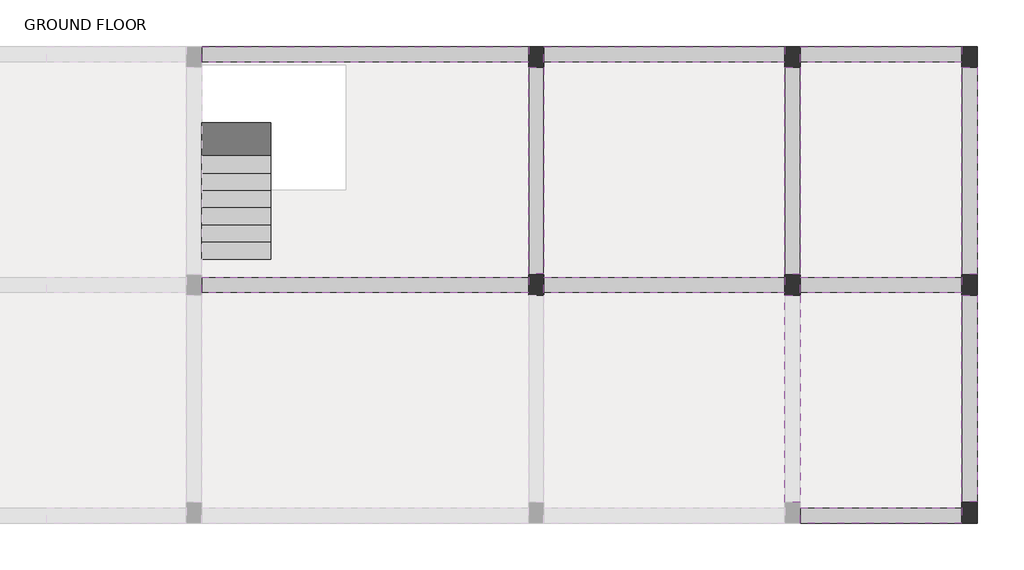
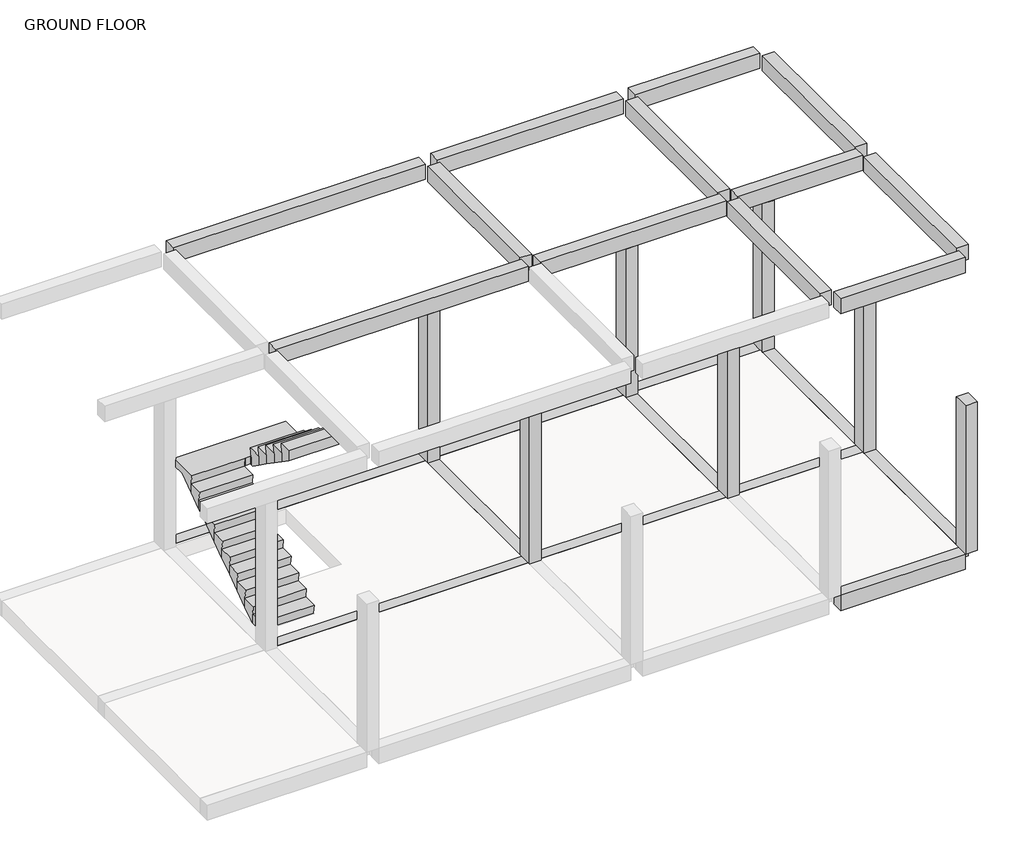
# One storey, part 2 of 2: 23 beams, 7 columns, 1 stair flight.
"""IFC4 building model written with IfcOpenShell, lengths in millimetres."""

from ifc_helpers import new_model, si_unit, frame, origin, place, context, project, spatial, polyline, outline, extrude, faceted_brep, element, save

model = new_model("IFC4")

# Units and contexts
model_context = context("Model", 3, world=origin())
ifc_project = project(units=[si_unit("LENGTHUNIT", "METRE", prefix="MILLI")], contexts=[model_context])

# Site, building, storey
site = spatial("IfcSite", under=ifc_project)
building = spatial("IfcBuilding", under=site)
storey = spatial("IfcBuildingStorey", under=building, Name="GROUND FLOOR", Elevation=0.0)

# Beams
placement = place(None, origin())
element("IfcBeam", 1, ObjectType="M_Concrete-Rectangular Beam : 100MM X 200MM", at=placement, inside=storey, context=model_context, shape_type="Brep", body=[
    faceted_brep([(9387.3931183, 2041.8765586, 0.0), (9387.3931183, 2270.4765586, 0.0), (7001.6931183, 2270.4765586, 0.0), (7001.6931183, 2041.8765586, 0.0), (9387.3931183, 2041.8765586, -304.8), (7001.6931183, 2041.8765586, -304.8), (9387.3931183, 2270.4765586, -304.8), (7001.6931183, 2270.4765586, -304.8), (7001.6931183, 2270.4765586, -300.0)], [[[0, 1, 2, 3]], [[4, 0, 3, 5]], [[6, 4, 5, 7]], [[1, 6, 7, 8, 2]], [[1, 0, 4, 6]], [[3, 2, 8, 7, 5]]]),
])
element("IfcBeam", 2, ObjectType="M_Concrete-Rectangular Beam : 100MM X 200MM", at=placement, inside=storey, context=model_context, shape_type="Brep", body=[
    faceted_brep([(2988.4931183, 8849.0765586, 0.0), (2988.4931183, 9077.6765586, 0.0), (-1837.5068817, 9077.6765586, 0.0), (-1837.5068817, 8849.0765586, 0.0), (2988.4931183, 8849.0765586, -304.8), (2988.4931183, 8849.0765586, -300.0), (-1837.5068817, 8849.0765586, -300.0), (-1837.5068817, 8849.0765586, -304.8), (2988.4931183, 9077.6765586, -304.8), (-1837.5068817, 9077.6765586, -304.8)], [[[0, 1, 2, 3]], [[4, 5, 0, 3, 6, 7]], [[8, 4, 7, 9]], [[1, 8, 9, 2]], [[1, 0, 5, 4, 8]], [[3, 2, 9, 7, 6]]]),
])
element("IfcBeam", 3, ObjectType="M_Concrete-Rectangular Beam : 100MM X 200MM", at=placement, inside=storey, context=model_context, shape_type="Brep", body=[
    faceted_brep([(6773.0931183, 8849.0765586, 0.0), (6773.0931183, 9077.6765586, 0.0), (3217.0931183, 9077.6765586, 0.0), (3217.0931183, 8849.0765586, 0.0), (6773.0931183, 8849.0765586, -304.8), (6773.0931183, 8849.0765586, -300.0), (3217.0931183, 8849.0765586, -300.0), (3217.0931183, 8849.0765586, -304.8), (6773.0931183, 9077.6765586, -304.8), (3217.0931183, 9077.6765586, -304.8)], [[[0, 1, 2, 3]], [[4, 5, 0, 3, 6, 7]], [[8, 4, 7, 9]], [[1, 8, 9, 2]], [[1, 0, 5, 4, 8]], [[3, 2, 9, 7, 6]]]),
])
element("IfcBeam", 4, ObjectType="M_Concrete-Rectangular Beam : 100MM X 200MM", at=placement, inside=storey, context=model_context, shape_type="Brep", body=[
    faceted_brep([(9387.3931183, 8849.0765586, 0.0), (9387.3931183, 9077.6765586, 0.0), (7001.6931183, 9077.6765586, 0.0), (7001.6931183, 8849.0765586, 0.0), (9387.3931183, 8849.0765586, -304.8), (7001.6931183, 8849.0765586, -300.0), (7001.6931183, 8849.0765586, -304.8), (9387.3931183, 9077.6765586, -304.8), (7001.6931183, 9077.6765586, -304.8)], [[[0, 1, 2, 3]], [[4, 0, 3, 5, 6]], [[7, 4, 6, 8]], [[1, 7, 8, 2]], [[1, 0, 4, 7]], [[3, 2, 8, 6, 5]]]),
])
element("IfcBeam", 5, ObjectType="M_Concrete-Rectangular Beam : 100MM X 200MM", at=placement, inside=storey, context=model_context, shape_type="SweptSolid", body=[
    extrude(outline(polyline([(9617.8931183, 2354.2765586), (9389.2931183, 2354.2765586), (9389.2931183, 5407.2180792), (9617.8931183, 5407.2180792), (9617.8931183, 2354.2765586)])), frame((0.0, 0.0, -304.8), z_axis=(0.0, 0.0, 1.0), x_axis=(1.0, 0.0, 0.0)), (0.0, 0.0, 1.0), 304.8),
])
element("IfcBeam", 6, ObjectType="M_Concrete-Rectangular Beam : 100MM X 200MM", at=placement, inside=storey, context=model_context, shape_type="SweptSolid", body=[
    extrude(outline(polyline([(9389.2931183, 8772.8765586), (9617.8931183, 8772.8765586), (9617.8931183, 5712.0180792), (9389.2931183, 5712.0180792), (9389.2931183, 8772.8765586)])), frame((0.0, 0.0, -304.8), z_axis=(0.0, 0.0, 1.0), x_axis=(1.0, 0.0, 0.0)), (0.0, 0.0, 1.0), 304.8),
])
element("IfcBeam", 7, ObjectType="M_Concrete-Rectangular Beam : 100MM X 200MM", at=placement, inside=storey, context=model_context, shape_type="Brep", body=[
    faceted_brep([(9389.2931183, 5445.3180792, 0.0), (9389.2931183, 5673.9180792, 0.0), (7001.6931183, 5673.9180792, 0.0), (7001.6931183, 5445.3180792, 0.0), (9389.2931183, 5673.9180792, -300.0), (9389.2931183, 5673.9180792, -304.8), (7001.6931183, 5673.9180792, -304.8), (7001.6931183, 5673.9180792, -300.0), (9389.2931183, 5445.3180792, -304.8), (7001.6931183, 5445.3180792, -304.8), (7001.6931183, 5445.3180792, -300.0), (9389.2931183, 5445.3180792, -300.0)], [[[0, 1, 2, 3]], [[2, 1, 4, 5, 6, 7]], [[5, 8, 9, 6]], [[0, 3, 10, 9, 8, 11]], [[1, 0, 11, 8, 5, 4]], [[3, 2, 7, 6, 9, 10]]]),
])
element("IfcBeam", 8, ObjectType="M_Concrete-Rectangular Beam : 100MM X 200MM", at=placement, inside=storey, context=model_context, shape_type="Brep", body=[
    faceted_brep([(6773.0931183, 5445.3180792, 0.0), (6773.0931183, 5673.9180792, 0.0), (3217.0931183, 5673.9180792, 0.0), (3217.0931183, 5445.3180792, 0.0), (6773.0931183, 5673.9180792, -300.0), (6773.0931183, 5673.9180792, -304.8), (3217.0931183, 5673.9180792, -304.8), (3217.0931183, 5673.9180792, -300.0), (6773.0931183, 5445.3180792, -304.8), (3217.0931183, 5445.3180792, -304.8), (3217.0931183, 5445.3180792, -300.0), (6773.0931183, 5445.3180792, -300.0)], [[[0, 1, 2, 3]], [[2, 1, 4, 5, 6, 7]], [[5, 8, 9, 6]], [[0, 3, 10, 9, 8, 11]], [[1, 0, 11, 8, 5, 4]], [[3, 2, 7, 6, 9, 10]]]),
])
element("IfcBeam", 9, ObjectType="M_Concrete-Rectangular Beam : 100MM X 200MM", at=placement, inside=storey, context=model_context, shape_type="Brep", body=[
    faceted_brep([(2988.4931183, 5445.3180792, 0.0), (2988.4931183, 5673.9180792, 0.0), (-1837.5068817, 5673.9180792, 0.0), (-1837.5068817, 5445.3180792, 0.0), (2988.4931183, 5673.9180792, -300.0), (2988.4931183, 5673.9180792, -304.8), (-1837.5068817, 5673.9180792, -304.8), (-1837.5068817, 5673.9180792, -300.0), (2988.4931183, 5445.3180792, -304.8), (-1837.5068817, 5445.3180792, -304.8), (-1837.5068817, 5445.3180792, -300.0), (2988.4931183, 5445.3180792, -300.0)], [[[0, 1, 2, 3]], [[2, 1, 4, 5, 6, 7]], [[5, 8, 9, 6]], [[0, 3, 10, 9, 8, 11]], [[1, 0, 11, 8, 5, 4]], [[3, 2, 7, 6, 9, 10]]]),
])
element("IfcBeam", 10, ObjectType="M_Concrete-Rectangular Beam : 100MM X 200MM", at=placement, inside=storey, context=model_context, shape_type="Brep", body=[
    faceted_brep([(7001.6931183, 8772.8765586, 0.0), (6773.0931183, 8772.8765586, 0.0), (6773.0931183, 5712.0180792, 0.0), (7001.6931183, 5712.0180792, 0.0), (7001.6931183, 5712.0180792, -300.0), (7001.6931183, 5712.0180792, -304.8), (7001.6931183, 8772.8765586, -304.8), (7001.6931183, 8772.8765586, -300.0), (6773.0931183, 8772.8765586, -304.8), (6773.0931183, 5712.0180792, -304.8), (6773.0931183, 8772.8765586, -300.0), (6773.0931183, 5712.0180792, -300.0)], [[[0, 1, 2, 3]], [[0, 3, 4, 5, 6, 7]], [[8, 6, 5, 9]], [[2, 1, 10, 8, 9, 11]], [[1, 0, 7, 6, 8, 10]], [[3, 2, 11, 9, 5, 4]]]),
])
element("IfcBeam", 11, ObjectType="M_Concrete-Rectangular Beam : 100MM X 200MM", at=placement, inside=storey, context=model_context, shape_type="Brep", body=[
    faceted_brep([(2988.4931183, 5719.6180792, 0.0), (3217.0931183, 5719.6180792, 0.0), (3217.0931183, 8772.8765586, 0.0), (2988.4931183, 8772.8765586, 0.0), (3217.0931183, 5719.6180792, -300.0), (3217.0931183, 5719.6180792, -304.8), (3217.0931183, 8772.8765586, -304.8), (3217.0931183, 8772.8765586, -300.0), (2988.4931183, 5719.6180792, -304.8), (2988.4931183, 8772.8765586, -304.8), (2988.4931183, 8772.8765586, -300.0), (2988.4931183, 5719.6180792, -300.0)], [[[0, 1, 2, 3]], [[2, 1, 4, 5, 6, 7]], [[5, 8, 9, 6]], [[0, 3, 10, 9, 8, 11]], [[8, 5, 4, 1, 0, 11]], [[3, 2, 7, 6, 9, 10]]]),
])
element("IfcBeam", 12, ObjectType="M_Concrete-Rectangular Beam : 100MM X 200MM", at=placement, inside=storey, context=model_context, shape_type="Brep", body=[
    faceted_brep([(9387.3931183, 2041.8765586, 6000.0), (9387.3931183, 2270.4765586, 6000.0), (7001.6931183, 2270.4765586, 6000.0), (7001.6931183, 2041.8765586, 6000.0), (9387.3931183, 2041.8765586, 5695.2), (7001.6931183, 2041.8765586, 5695.2), (9387.3931183, 2270.4765586, 5695.2), (7001.6931183, 2270.4765586, 5695.2), (7001.6931183, 2270.4765586, 5700.0)], [[[0, 1, 2, 3]], [[4, 0, 3, 5]], [[6, 4, 5, 7]], [[1, 6, 7, 8, 2]], [[1, 0, 4, 6]], [[3, 2, 8, 7, 5]]]),
])
element("IfcBeam", 13, ObjectType="M_Concrete-Rectangular Beam : 100MM X 200MM", at=placement, inside=storey, context=model_context, shape_type="Brep", body=[
    faceted_brep([(2988.4931183, 8849.0765586, 6000.0), (2988.4931183, 9077.6765586, 6000.0), (-1837.5068817, 9077.6765586, 6000.0), (-1837.5068817, 8849.0765586, 6000.0), (2988.4931183, 8849.0765586, 5695.2), (2988.4931183, 8849.0765586, 5700.0), (-1837.5068817, 8849.0765586, 5700.0), (-1837.5068817, 8849.0765586, 5695.2), (2988.4931183, 9077.6765586, 5695.2), (-1837.5068817, 9077.6765586, 5695.2)], [[[0, 1, 2, 3]], [[4, 5, 0, 3, 6, 7]], [[8, 4, 7, 9]], [[1, 8, 9, 2]], [[1, 0, 5, 4, 8]], [[3, 2, 9, 7, 6]]]),
])
element("IfcBeam", 14, ObjectType="M_Concrete-Rectangular Beam : 100MM X 200MM", at=placement, inside=storey, context=model_context, shape_type="Brep", body=[
    faceted_brep([(6773.0931183, 8849.0765586, 6000.0), (6773.0931183, 9077.6765586, 6000.0), (3217.0931183, 9077.6765586, 6000.0), (3217.0931183, 8849.0765586, 6000.0), (6773.0931183, 8849.0765586, 5695.2), (6773.0931183, 8849.0765586, 5700.0), (3217.0931183, 8849.0765586, 5700.0), (3217.0931183, 8849.0765586, 5695.2), (6773.0931183, 9077.6765586, 5695.2), (3217.0931183, 9077.6765586, 5695.2)], [[[0, 1, 2, 3]], [[4, 5, 0, 3, 6, 7]], [[8, 4, 7, 9]], [[1, 8, 9, 2]], [[1, 0, 5, 4, 8]], [[3, 2, 9, 7, 6]]]),
])
element("IfcBeam", 15, ObjectType="M_Concrete-Rectangular Beam : 100MM X 200MM", at=placement, inside=storey, context=model_context, shape_type="Brep", body=[
    faceted_brep([(9387.3931183, 8849.0765586, 6000.0), (9387.3931183, 9077.6765586, 6000.0), (7001.6931183, 9077.6765586, 6000.0), (7001.6931183, 8849.0765586, 6000.0), (9387.3931183, 8849.0765586, 5695.2), (7001.6931183, 8849.0765586, 5700.0), (7001.6931183, 8849.0765586, 5695.2), (9387.3931183, 9077.6765586, 5695.2), (7001.6931183, 9077.6765586, 5695.2)], [[[0, 1, 2, 3]], [[4, 0, 3, 5, 6]], [[7, 4, 6, 8]], [[1, 7, 8, 2]], [[1, 0, 4, 7]], [[3, 2, 8, 6, 5]]]),
])
element("IfcBeam", 16, ObjectType="M_Concrete-Rectangular Beam : 100MM X 200MM", at=placement, inside=storey, context=model_context, shape_type="SweptSolid", body=[
    extrude(outline(polyline([(9617.8931183, 2354.2765586), (9389.2931183, 2354.2765586), (9389.2931183, 5407.2180792), (9617.8931183, 5407.2180792), (9617.8931183, 2354.2765586)])), frame((0.0, 0.0, 5695.2), z_axis=(0.0, 0.0, 1.0), x_axis=(1.0, 0.0, 0.0)), (0.0, 0.0, 1.0), 304.8),
])
element("IfcBeam", 17, ObjectType="M_Concrete-Rectangular Beam : 100MM X 200MM", at=placement, inside=storey, context=model_context, shape_type="SweptSolid", body=[
    extrude(outline(polyline([(9389.2931183, 8772.8765586), (9617.8931183, 8772.8765586), (9617.8931183, 5712.0180792), (9389.2931183, 5712.0180792), (9389.2931183, 8772.8765586)])), frame((0.0, 0.0, 5695.2), z_axis=(0.0, 0.0, 1.0), x_axis=(1.0, 0.0, 0.0)), (0.0, 0.0, 1.0), 304.8),
])
element("IfcBeam", 18, ObjectType="M_Concrete-Rectangular Beam : 100MM X 200MM", at=placement, inside=storey, context=model_context, shape_type="Brep", body=[
    faceted_brep([(7001.6931183, 5445.3180792, 6000.0), (9389.2931183, 5445.3180792, 6000.0), (9389.2931183, 5673.9180792, 6000.0), (7001.6931183, 5673.9180792, 6000.0), (9389.2931183, 5673.9180792, 5700.0), (9389.2931183, 5673.9180792, 5695.2), (7001.6931183, 5673.9180792, 5695.2), (7001.6931183, 5673.9180792, 5700.0), (9389.2931183, 5445.3180792, 5695.2), (7001.6931183, 5445.3180792, 5695.2), (7001.6931183, 5445.3180792, 5700.0), (9389.2931183, 5445.3180792, 5700.0)], [[[0, 1, 2, 3]], [[3, 2, 4, 5, 6, 7]], [[5, 8, 9, 6]], [[1, 0, 10, 9, 8, 11]], [[5, 4, 2, 1, 11, 8]], [[0, 3, 7, 6, 9, 10]]]),
])
element("IfcBeam", 19, ObjectType="M_Concrete-Rectangular Beam : 100MM X 200MM", at=placement, inside=storey, context=model_context, shape_type="Brep", body=[
    faceted_brep([(3217.0931183, 5445.3180792, 6000.0), (6773.0931183, 5445.3180792, 6000.0), (6773.0931183, 5673.9180792, 6000.0), (3217.0931183, 5673.9180792, 6000.0), (6773.0931183, 5673.9180792, 5700.0), (6773.0931183, 5673.9180792, 5695.2), (3217.0931183, 5673.9180792, 5695.2), (3217.0931183, 5673.9180792, 5700.0), (6773.0931183, 5445.3180792, 5695.2), (3217.0931183, 5445.3180792, 5695.2), (3217.0931183, 5445.3180792, 5700.0), (6773.0931183, 5445.3180792, 5700.0)], [[[0, 1, 2, 3]], [[3, 2, 4, 5, 6, 7]], [[5, 8, 9, 6]], [[1, 0, 10, 9, 8, 11]], [[2, 1, 11, 8, 5, 4]], [[0, 3, 7, 6, 9, 10]]]),
])
element("IfcBeam", 20, ObjectType="M_Concrete-Rectangular Beam : 100MM X 200MM", at=placement, inside=storey, context=model_context, shape_type="Brep", body=[
    faceted_brep([(-1837.5068817, 5445.3180792, 6000.0), (2988.4931183, 5445.3180792, 6000.0), (2988.4931183, 5673.9180792, 6000.0), (-1837.5068817, 5673.9180792, 6000.0), (2988.4931183, 5673.9180792, 5700.0), (2988.4931183, 5673.9180792, 5695.2), (-1837.5068817, 5673.9180792, 5695.2), (-1837.5068817, 5673.9180792, 5700.0), (2988.4931183, 5445.3180792, 5695.2), (-1837.5068817, 5445.3180792, 5695.2), (-1837.5068817, 5445.3180792, 5700.0), (2988.4931183, 5445.3180792, 5700.0)], [[[0, 1, 2, 3]], [[3, 2, 4, 5, 6, 7]], [[5, 8, 9, 6]], [[1, 0, 10, 9, 8, 11]], [[2, 1, 11, 8, 5, 4]], [[0, 3, 7, 6, 9, 10]]]),
])
element("IfcBeam", 21, ObjectType="M_Concrete-Rectangular Beam : 100MM X 200MM", at=placement, inside=storey, context=model_context, shape_type="SweptSolid", body=[
    extrude(outline(polyline([(6773.0931183, 5407.2180792), (7001.6931183, 5407.2180792), (7001.6931183, 2346.6765586), (6773.0931183, 2346.6765586), (6773.0931183, 5407.2180792)])), frame((0.0, 0.0, 5695.2), z_axis=(0.0, 0.0, 1.0), x_axis=(1.0, 0.0, 0.0)), (0.0, 0.0, 1.0), 304.8),
])
element("IfcBeam", 22, ObjectType="M_Concrete-Rectangular Beam : 100MM X 200MM", at=placement, inside=storey, context=model_context, shape_type="SweptSolid", body=[
    extrude(outline(polyline([(6773.0931183, 8772.8765586), (7001.6931183, 8772.8765586), (7001.6931183, 5712.0180792), (6773.0931183, 5712.0180792), (6773.0931183, 8772.8765586)])), frame((0.0, 0.0, 5695.2), z_axis=(0.0, 0.0, 1.0), x_axis=(1.0, 0.0, 0.0)), (0.0, 0.0, 1.0), 304.8),
])
element("IfcBeam", 23, ObjectType="M_Concrete-Rectangular Beam : 100MM X 200MM", at=placement, inside=storey, context=model_context, shape_type="Brep", body=[
    faceted_brep([(2988.4931183, 5719.6180792, 6000.0), (3217.0931183, 5719.6180792, 6000.0), (3217.0931183, 8772.8765586, 6000.0), (2988.4931183, 8772.8765586, 6000.0), (3217.0931183, 5719.6180792, 5700.0), (3217.0931183, 5719.6180792, 5695.2), (3217.0931183, 8772.8765586, 5695.2), (2988.4931183, 5719.6180792, 5695.2), (2988.4931183, 8772.8765586, 5695.2), (2988.4931183, 5719.6180792, 5700.0)], [[[0, 1, 2, 3]], [[1, 4, 5, 6, 2]], [[5, 7, 8, 6]], [[7, 9, 0, 3, 8]], [[7, 5, 4, 1, 0, 9]], [[3, 2, 6, 8]]]),
])

# Columns
element("IfcColumn", 24, ObjectType="M_Concrete-Rectangular-Column : 9\" X 1' COLUMNS", at=placement, inside=storey, context=model_context, shape_type="Brep", body=[
    faceted_brep([(9617.8931183, 9077.6765586, 0.0), (9617.8931183, 8772.8765586, 0.0), (9389.2931183, 8772.8765586, 0.0), (9389.2931183, 9077.6765586, 0.0), (9617.8931183, 9077.6765586, 3000.0), (9617.8931183, 8772.8765586, 3000.0), (9389.2931183, 8772.8765586, 3000.0), (9389.2931183, 8849.0765586, 3000.0), (9389.2931183, 9077.6765586, 3000.0)], [[[0, 1, 2, 3]], [[4, 5, 1, 0]], [[5, 6, 2, 1]], [[6, 7, 8, 3, 2]], [[8, 4, 0, 3]], [[4, 8, 7, 6, 5]]]),
])
element("IfcColumn", 25, ObjectType="M_Concrete-Rectangular-Column : 9\" X 1' COLUMNS", at=placement, inside=storey, context=model_context, shape_type="Brep", body=[
    faceted_brep([(9617.8931183, 5712.0180792, 0.0), (9617.8931183, 5407.2180792, 0.0), (9389.2931183, 5407.2180792, 0.0), (9389.2931183, 5712.0180792, 0.0), (9617.8931183, 5712.0180792, 3000.0), (9617.8931183, 5407.2180792, 3000.0), (9389.2931183, 5407.2180792, 3000.0), (9389.2931183, 5445.3180792, 3000.0), (9389.2931183, 5673.9180792, 3000.0), (9389.2931183, 5712.0180792, 3000.0)], [[[0, 1, 2, 3]], [[4, 5, 1, 0]], [[5, 6, 2, 1]], [[6, 7, 8, 9, 3, 2]], [[9, 4, 0, 3]], [[4, 9, 8, 7, 6, 5]]]),
])
element("IfcColumn", 26, ObjectType="M_Concrete-Rectangular-Column : 9\" X 1' COLUMNS", at=placement, inside=storey, context=model_context, shape_type="Brep", body=[
    faceted_brep([(9617.8931183, 2346.6765586, 0.0), (9617.8931183, 2041.8765586, 0.0), (9389.2931183, 2041.8765586, 0.0), (9389.2931183, 2346.6765586, 0.0), (9617.8931183, 2346.6765586, 3000.0), (9617.8931183, 2041.8765586, 3000.0), (9389.2931183, 2041.8765586, 3000.0), (9389.2931183, 2270.4765586, 3000.0), (9389.2931183, 2346.6765586, 3000.0)], [[[0, 1, 2, 3]], [[4, 5, 1, 0]], [[5, 6, 2, 1]], [[6, 7, 8, 3, 2]], [[8, 4, 0, 3]], [[4, 8, 7, 6, 5]]]),
])
element("IfcColumn", 27, ObjectType="M_Concrete-Rectangular-Column : 9\" X 1' COLUMNS", at=placement, inside=storey, context=model_context, shape_type="Brep", body=[
    faceted_brep([(7001.6931183, 9077.6765586, 0.0), (7001.6931183, 8772.8765586, 0.0), (6773.0931183, 8772.8765586, 0.0), (6773.0931183, 9077.6765586, 0.0), (7001.6931183, 9077.6765586, 3000.0), (7001.6931183, 8849.0765586, 3000.0), (7001.6931183, 8772.8765586, 3000.0), (7001.6931183, 8772.8765586, 2700.0), (6773.0931183, 8772.8765586, 3000.0), (6773.0931183, 8772.8765586, 2700.0), (6773.0931183, 8849.0765586, 3000.0), (6773.0931183, 9077.6765586, 3000.0)], [[[0, 1, 2, 3]], [[1, 0, 4, 5, 6, 7]], [[2, 1, 7, 6, 8, 9]], [[3, 2, 9, 8, 10, 11]], [[0, 3, 11, 4]], [[8, 6, 5, 4, 11, 10]]]),
])
element("IfcColumn", 28, ObjectType="M_Concrete-Rectangular-Column : 9\" X 1' COLUMNS", at=placement, inside=storey, context=model_context, shape_type="Brep", body=[
    faceted_brep([(7001.6931183, 5712.0180792, 0.0), (7001.6931183, 5407.2180792, 0.0), (6773.0931183, 5407.2180792, 0.0), (6773.0931183, 5712.0180792, 0.0), (7001.6931183, 5712.0180792, 2700.0), (7001.6931183, 5712.0180792, 3000.0), (7001.6931183, 5673.9180792, 3000.0), (7001.6931183, 5445.3180792, 3000.0), (7001.6931183, 5407.2180792, 3000.0), (7001.6931183, 5407.2180792, 2700.0), (6773.0931183, 5407.2180792, 3000.0), (6773.0931183, 5407.2180792, 2700.0), (6773.0931183, 5445.3180792, 3000.0), (6773.0931183, 5673.9180792, 3000.0), (6773.0931183, 5712.0180792, 3000.0), (6773.0931183, 5712.0180792, 2700.0)], [[[0, 1, 2, 3]], [[1, 0, 4, 5, 6, 7, 8, 9]], [[2, 1, 9, 8, 10, 11]], [[3, 2, 11, 10, 12, 13, 14, 15]], [[0, 3, 15, 14, 5, 4]], [[10, 8, 7, 6, 5, 14, 13, 12]]]),
])
element("IfcColumn", 29, ObjectType="M_Concrete-Rectangular-Column : 9\" X 1' COLUMNS", at=placement, inside=storey, context=model_context, shape_type="Brep", body=[
    faceted_brep([(3217.0931183, 9077.6765586, 0.0), (3217.0931183, 8772.8765586, 0.0), (2988.4931183, 8772.8765586, 0.0), (2988.4931183, 9077.6765586, 0.0), (3217.0931183, 9077.6765586, 3000.0), (3217.0931183, 8849.0765586, 3000.0), (3217.0931183, 8772.8765586, 3000.0), (3217.0931183, 8772.8765586, 2700.0), (2988.4931183, 8772.8765586, 3000.0), (2988.4931183, 8772.8765586, 2700.0), (2988.4931183, 8849.0765586, 3000.0), (2988.4931183, 9077.6765586, 3000.0)], [[[0, 1, 2, 3]], [[1, 0, 4, 5, 6, 7]], [[2, 1, 7, 6, 8, 9]], [[3, 2, 9, 8, 10, 11]], [[0, 3, 11, 4]], [[8, 6, 5, 4, 11, 10]]]),
])
element("IfcColumn", 30, ObjectType="M_Concrete-Rectangular-Column : 9\" X 1' COLUMNS", at=placement, inside=storey, context=model_context, shape_type="Brep", body=[
    faceted_brep([(3217.0931183, 5712.0180792, 0.0), (3217.0931183, 5407.2180792, 0.0), (2988.4931183, 5407.2180792, 0.0), (2988.4931183, 5712.0180792, 0.0), (3217.0931183, 5712.0180792, 2700.0), (3217.0931183, 5712.0180792, 3000.0), (3217.0931183, 5673.9180792, 3000.0), (3217.0931183, 5445.3180792, 3000.0), (3217.0931183, 5407.2180792, 3000.0), (3217.0931183, 5407.2180792, 2700.0), (2988.4931183, 5407.2180792, 3000.0), (2988.4931183, 5407.2180792, 2700.0), (2988.4931183, 5445.3180792, 3000.0), (2988.4931183, 5673.9180792, 3000.0), (2988.4931183, 5712.0180792, 3000.0), (2988.4931183, 5712.0180792, 2700.0)], [[[0, 1, 2, 3]], [[1, 0, 4, 5, 6, 7, 8, 9]], [[2, 1, 9, 8, 10, 11]], [[3, 2, 11, 10, 12, 13, 14, 15]], [[0, 3, 15, 14, 5, 4]], [[10, 8, 7, 6, 5, 14, 13, 12]]]),
])

# Stair flight
element("IfcStairFlight", 31, ObjectType="25 mm Nosing", at=placement, inside=storey, context=model_context, shape_type="Brep", body=[
    faceted_brep([(-1837.5068817, 5940.7765586, 176.4705882), (-821.5068817, 5940.7765586, 176.4705882), (-821.5068817, 6219.7765586, 176.4705882), (-1837.5068817, 6219.7765586, 176.4705882), (-1837.5068817, 6219.7765586, 0.0), (-1837.5068817, 5965.7765586, 0.0), (-821.5068817, 5965.7765586, 0.0), (-821.5068817, 6219.7765586, 0.0), (-1837.5068817, 6194.7765586, 352.9411765), (-821.5068817, 6194.7765586, 352.9411765), (-821.5068817, 6473.7765586, 352.9411765), (-1837.5068817, 6473.7765586, 352.9411765), (-1837.5068817, 6473.7765586, 170.2919269), (-1837.5068817, 6228.6697118, 0.0), (-821.5068817, 6228.6697118, 0.0), (-821.5068817, 6473.7765586, 170.2919269), (-1837.5068817, 6448.7765586, 529.4117647), (-821.5068817, 6448.7765586, 529.4117647), (-821.5068817, 6727.7765586, 529.4117647), (-1837.5068817, 6727.7765586, 529.4117647), (-1837.5068817, 6727.7765586, 346.7625151), (-821.5068817, 6727.7765586, 346.7625151), (-1837.5068817, 6702.7765586, 705.8823529), (-821.5068817, 6702.7765586, 705.8823529), (-821.5068817, 6981.7765586, 705.8823529), (-1837.5068817, 6981.7765586, 705.8823529), (-1837.5068817, 6981.7765586, 523.2331034), (-821.5068817, 6981.7765586, 523.2331034), (-1837.5068817, 6956.7765586, 882.3529412), (-821.5068817, 6956.7765586, 882.3529412), (-821.5068817, 7235.7765586, 882.3529412), (-1837.5068817, 7235.7765586, 882.3529412), (-1837.5068817, 7235.7765586, 699.7036916), (-821.5068817, 7235.7765586, 699.7036916), (-1837.5068817, 7210.7765586, 1058.8235294), (-821.5068817, 7210.7765586, 1058.8235294), (-821.5068817, 7489.7765586, 1058.8235294), (-1837.5068817, 7489.7765586, 1058.8235294), (-1837.5068817, 7489.7765586, 876.1742799), (-821.5068817, 7489.7765586, 876.1742799), (-1837.5068817, 7464.7765586, 1235.2941176), (-821.5068817, 7464.7765586, 1235.2941176), (-821.5068817, 7743.7765586, 1235.2941176), (-1837.5068817, 7743.7765586, 1235.2941176), (-1837.5068817, 7743.7765586, 1052.6448681), (-821.5068817, 7743.7765586, 1052.6448681), (-1837.5068817, 7718.7765586, 1411.7647059), (-821.5068817, 7718.7765586, 1411.7647059), (-821.5068817, 7997.7765586, 1411.7647059), (-1837.5068817, 7997.7765586, 1411.7647059), (-1837.5068817, 7997.7765586, 1229.1154563), (-821.5068817, 7997.7765586, 1229.1154563), (-1837.5068817, 7972.7765586, 1588.2352941), (-821.5068817, 7972.7765586, 1588.2352941), (-821.5068817, 8251.7765586, 1588.2352941), (-1837.5068817, 8251.7765586, 1588.2352941), (-1837.5068817, 8251.7765586, 1405.5860446), (-821.5068817, 8552.7697118, 1614.7058824), (-821.5068817, 8248.0265586, 1614.7058824), (296.0931183, 8201.7765586, 1764.7058824), (296.0931183, 8810.9765586, 1764.7058824), (-1837.5068817, 8810.9765586, 1764.7058824), (-1837.5068817, 8552.7697118, 1764.7058824), (-1837.5068817, 8226.7765586, 1764.7058824), (-821.5068817, 8226.7765586, 1764.7058824), (-719.9068817, 8226.7765586, 1764.7058824), (-719.9068817, 8201.7765586, 1764.7058824), (296.0931183, 8201.7765586, 1614.7058824), (296.0931183, 8810.9765586, 1614.7058824), (-1837.5068817, 8810.9765586, 1614.7058824), (-1837.5068817, 8552.7697118, 1614.7058824), (-821.5068817, 8226.7765586, 1614.7058824), (-719.9068817, 8226.7765586, 1614.7058824), (-719.9068817, 8201.7765586, 1614.7058824), (296.0931183, 8226.7765586, 1941.1764706), (-719.9068817, 8226.7765586, 1941.1764706), (-719.9068817, 8154.7834054, 1941.1764706), (-719.9068817, 7947.7765586, 1941.1764706), (296.0931183, 7947.7765586, 1941.1764706), (296.0931183, 8154.7834054, 1941.1764706), (296.0931183, 7947.7765586, 1758.527221), (296.0931183, 8154.7834054, 1614.7058824), (-719.9068817, 8154.7834054, 1614.7058824), (-719.9068817, 7947.7765586, 1758.527221), (296.0931183, 7972.7765586, 2117.6470588), (-719.9068817, 7972.7765586, 2117.6470588), (-719.9068817, 7693.7765586, 2117.6470588), (296.0931183, 7693.7765586, 2117.6470588), (296.0931183, 7693.7765586, 1934.9978093), (-719.9068817, 7693.7765586, 1934.9978093), (296.0931183, 7718.7765586, 2294.1176471), (-719.9068817, 7718.7765586, 2294.1176471), (-719.9068817, 7439.7765586, 2294.1176471), (296.0931183, 7439.7765586, 2294.1176471), (296.0931183, 7439.7765586, 2111.4683975), (-719.9068817, 7439.7765586, 2111.4683975), (296.0931183, 7464.7765586, 2470.5882353), (-719.9068817, 7464.7765586, 2470.5882353), (-719.9068817, 7185.7765586, 2470.5882353), (296.0931183, 7185.7765586, 2470.5882353), (296.0931183, 7185.7765586, 2287.9389857), (-719.9068817, 7185.7765586, 2287.9389857), (296.0931183, 7210.7765586, 2647.0588235), (-719.9068817, 7210.7765586, 2647.0588235), (-719.9068817, 6956.7765586, 2647.0588235), (296.0931183, 6956.7765586, 2647.0588235), (296.0931183, 6956.7765586, 2447.0404216), (-719.9068817, 6956.7765586, 2447.0404216)], [[[0, 1, 2, 3]], [[0, 3, 4, 5]], [[2, 1, 6, 7]], [[8, 9, 10, 11]], [[4, 3, 8, 11, 12, 13]], [[2, 7, 14, 15, 10, 9]], [[16, 17, 18, 19]], [[16, 19, 20, 12, 11]], [[18, 17, 10, 15, 21]], [[22, 23, 24, 25]], [[22, 25, 26, 20, 19]], [[24, 23, 18, 21, 27]], [[28, 29, 30, 31]], [[28, 31, 32, 26, 25]], [[30, 29, 24, 27, 33]], [[34, 35, 36, 37]], [[34, 37, 38, 32, 31]], [[36, 35, 30, 33, 39]], [[40, 41, 42, 43]], [[40, 43, 44, 38, 37]], [[42, 41, 36, 39, 45]], [[46, 47, 48, 49]], [[46, 49, 50, 44, 43]], [[48, 47, 42, 45, 51]], [[52, 53, 54, 55]], [[52, 55, 56, 50, 49]], [[53, 48, 51, 57, 58, 54]], [[59, 60, 61, 62, 63, 64, 65, 66]], [[60, 59, 67, 68]], [[61, 60, 68, 69]], [[55, 63, 62, 61, 69, 70, 56]], [[64, 58, 71]], [[65, 64, 71, 72]], [[66, 65, 72, 73]], [[74, 75, 76, 77, 78, 79]], [[59, 74, 79, 78, 80, 81, 67]], [[75, 66, 73, 82, 83, 77, 76]], [[84, 85, 86, 87]], [[84, 87, 88, 80, 78]], [[86, 85, 77, 83, 89]], [[90, 91, 92, 93]], [[90, 93, 94, 88, 87]], [[92, 91, 86, 89, 95]], [[96, 97, 98, 99]], [[96, 99, 100, 94, 93]], [[98, 97, 92, 95, 101]], [[1, 0, 5, 6]], [[3, 2, 9, 8]], [[11, 10, 17, 16]], [[19, 18, 23, 22]], [[25, 24, 29, 28]], [[31, 30, 35, 34]], [[37, 36, 41, 40]], [[43, 42, 47, 46]], [[49, 48, 53, 52]], [[55, 54, 58, 64, 63]], [[59, 66, 75, 74]], [[78, 77, 85, 84]], [[87, 86, 91, 90]], [[93, 92, 97, 96]], [[102, 103, 104, 105]], [[102, 105, 106, 100, 99]], [[104, 103, 98, 101, 107]], [[105, 104, 107, 106]], [[99, 98, 103, 102]], [[5, 4, 13, 14, 7, 6]], [[70, 57, 51, 45, 39, 33, 27, 21, 15, 14, 13, 12, 20, 26, 32, 38, 44, 50, 56]], [[57, 70, 69, 68, 67, 81, 82, 73, 72, 71, 58]], [[82, 81, 80, 88, 94, 100, 106, 107, 101, 95, 89, 83]]]),
])

save(model, "model.ifc")

# Revit data of these elements
# Type "M_Concrete-Rectangular Beam : 100MM X 200MM"
#   Length [instance default] = 1524 mm
#   b = 228.6 mm
#   h = 304.8 mm
#   Structural Material [instance default] = Concrete, Cast-in-Place gray
#   Assembly Code = ""
# Type "M_Concrete-Rectangular-Column : 9\" X 1' COLUMNS"
#   b = 228.6 mm
#   h = 304.8 mm
#   Structural Material [instance default] = Concrete, Cast-in-Place gray
# Elements 1, 2, 3, 4, 5, 6, 7, 8, 9, 10, 11, 12, 13, 14, 15, 16, 17, 18, 19, 20, 21, 22, 23 (IfcBeam, "M_Concrete-Rectangular Beam : 100MM X 200MM")
#   Structural Material = Concrete, Cast-in-Place gray
#   Phase Created = New Construction
#   Materials on its faces: "Concrete, Cast-in-Place gray"
# Elements 24, 25, 26, 27, 28, 29, 30 (IfcColumn, "M_Concrete-Rectangular-Column : 9\" X 1' COLUMNS")
#   Structural Material = Concrete, Cast-in-Place gray
#   Phase Created = New Construction
#   Materials on its faces: "Concrete, Cast-in-Place gray"
# Element 31 (IfcStairFlight, "25 mm Nosing")
#   Phase Created = New Construction
#   Materials on its faces: "Concrete, Cast In Situ"
# Materials
#   "Concrete, Cast-in-Place gray": class "Concrete", colour RGB 192 192 192, transparency 0, Description = "Cast-in-place concrete", Cost = 0
#   "Concrete, Cast In Situ": class "Concrete", colour RGB 192 192 192, transparency 0, Description = "physical material", Cost = 0
